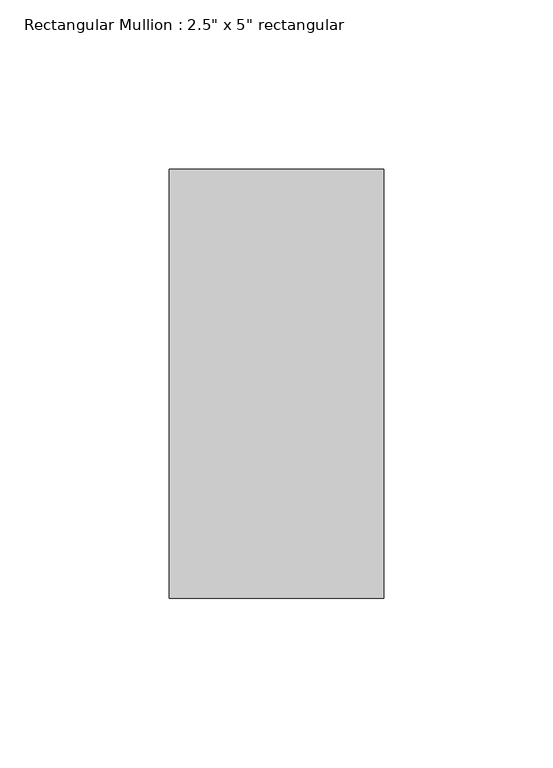
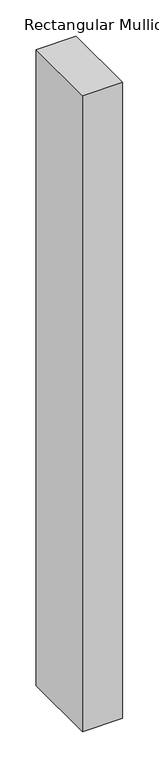
"""IFC4 building model written with IfcOpenShell, lengths in millimetres: member geometry."""

from ifc_helpers import new_model, si_unit, frame, origin, place, context, project, spatial, polyline, outline, extrude, source, transform, mapped, element, save


def member_a715cb85(model_context):
    return source(origin(), model_context, "Body", "SweptSolid", [
        extrude(outline(polyline([(31.75, 63.5), (31.75, -63.5), (-31.75, -63.5), (-31.75, 63.5), (31.75, 63.5)])), frame((0.0, 0.0, -1066.8), z_axis=(0.0, 0.0, 1.0), x_axis=(1.0, 0.0, 0.0)), (0.0, 0.0, 1.0), 1066.8),
    ])


if __name__ == "__main__":
    model = new_model("IFC4")
    model_context = context("Model", 3, world=origin())
    ifc_project = project(units=[si_unit("LENGTHUNIT", "METRE", prefix="MILLI")], contexts=[model_context])
    site = spatial("IfcSite", under=ifc_project)
    building = spatial("IfcBuilding", under=site)
    placement = place(None, origin())
    member_shape = member_a715cb85(model_context)
    element("IfcMember", 1, ObjectType="Rectangular Mullion : 2.5\" x 5\" rectangular", at=placement, inside=building, context=model_context, shape_type="MappedRepresentation", body=[
        mapped(member_shape, transform((0.0, 0.0, 0.0), x_axis=(1.0, 0.0, 0.0), y_axis=(0.0, 1.0, 0.0), z_axis=(0.0, 0.0, 1.0))),
    ])
    save(model, "model.ifc")

# Revit data of these elements
# Type "Rectangular Mullion : 2.5\" x 5\" rectangular"
#   built-in parameter 1007304 = 0.416667 (stored number, unit not read)
#   built-in parameter 1007301 = 0.104167 (stored number, unit not read)
#   built-in parameter 1007300 = 0.104167 (stored number, unit not read)
# Element 1 (IfcMember, "Rectangular Mullion : 2.5\" x 5\" rectangular")
#   Materials on its faces: "Aluminum"
# Materials
#   "Aluminum": class "Metal", colour RGB 247 247 247, transparency 0, Description = "Aluminum 6061", Cost = 0
